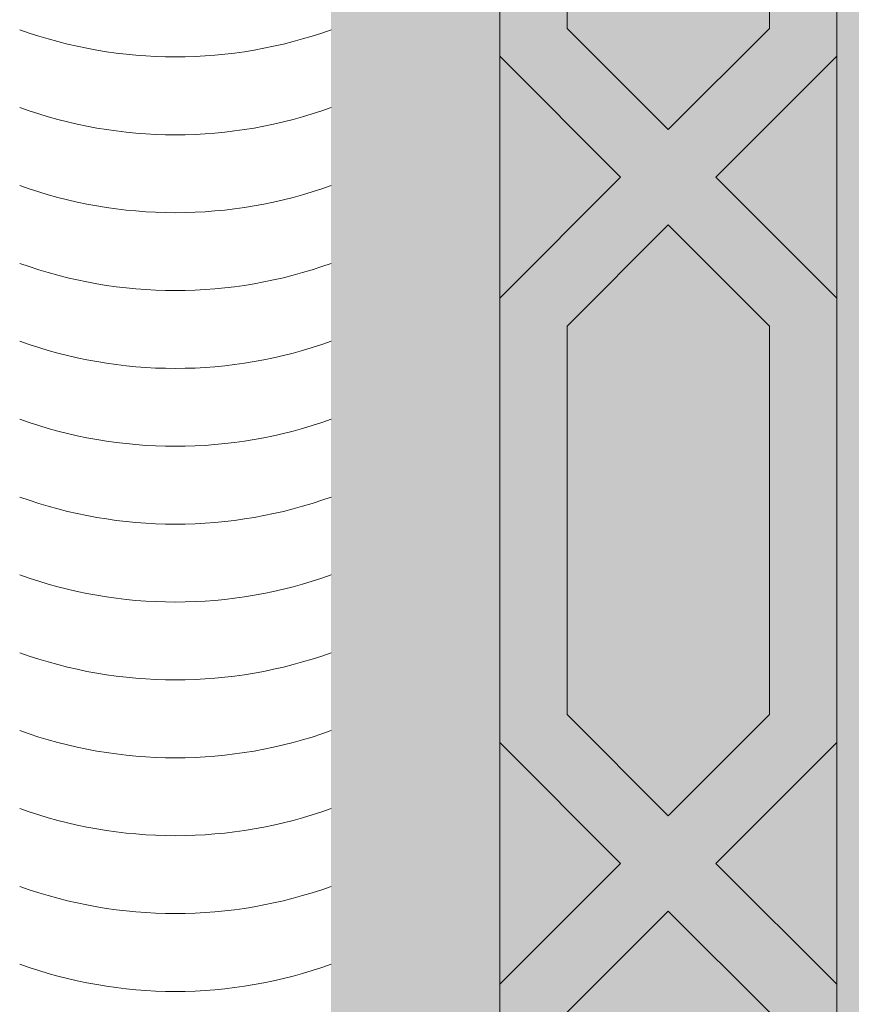
# Model space of a CAD drawing. Units: inches. Extents: x 844 to 2234, y 346 to 1084.
# Tile 58 of 93: x 1861.148 to 1864.294, y 706.48 to 710.205. Entities that reach past the tile are written whole.
import ezdxf

# ---------------------------------------------------------------- set-up
doc = ezdxf.new("R2010")
doc.units = ezdxf.units.IN
doc.header["$MEASUREMENT"] = 0
doc.layers.add('furniture', color=8, linetype='Continuous', lineweight=18)
doc.layers.add('RA-AP-01$0$INT', color=35, linetype='Continuous', lineweight=5)
doc.layers.add('RA-AP-01$0$FURN', color=3, linetype='Continuous')

# ---------------------------------------------------------------- blocks, each defined once
blk = doc.blocks.new('A$C18D01794')
at = {"layer": 'RA-AP-01$0$INT'}
h = blk.add_hatch(color=256, dxfattribs=at)
h.paths.add_polyline_path([(4.355206456958071, -6.156712009588037), (4.355206456958071, -8.056712009588038), (5.455206456958072, -8.056712009588038), (5.455206456958072, -6.156712009588037)])
h.paths.add_polyline_path([(4.405206456958072, -8.006712009588039), (4.405206456958072, -6.206712009588038), (5.405206456958072, -6.206712009588038), (5.405206456958072, -8.006712009588039)], flags=16)
h = blk.add_hatch(color=256, dxfattribs=at)
h.paths.add_polyline_path([(4.505206456958071, -7.585498806127123), (4.46934859260189, -7.549640941759413), (4.505206456958071, -7.513783077414768), (4.505206456958071, -7.381963272220687), (4.469348592616735, -7.346105407867824), (4.505206456958071, -7.310247543514964), (4.505206456958071, -7.178427738324996), (4.469348592586679, -7.142569873965138), (4.505206456952245, -7.106712009588038), (4.476922185709333, -7.106712009588038), (4.455206456960671, -7.128427738343681), (4.433490728198047, -7.106712009588038), (4.405206456946033, -7.106712009588036), (4.441064321339216, -7.142569873969684), (4.40520645695807, -7.178427738362358), (4.405206456958072, -7.310247543472698), (4.441064321364728, -7.346105407867826), (4.40520645695807, -7.381963272262947), (4.40520645695807, -7.513783077378263), (4.441064321354429, -7.549640941786153), (4.405206456958072, -7.585498806170974), (4.405206456958072, -7.717318611286652), (4.441064321333084, -7.753176475673194), (4.405206456958072, -7.789034340036673), (4.405206456958072, -8.006712009588039), (4.644348592588106, -8.006712009588039), (4.680206456964639, -7.970854145211967), (4.716064321341165, -8.006712009588039), (4.869348592586113, -8.006712009588039), (4.905206456964143, -7.970854145210465), (4.941064321342174, -8.006712009588039), (5.094348592587118, -8.006712009588037), (5.130206456963649, -7.970854145211967), (5.166064321340178, -8.006712009588039), (5.405206456958072, -8.006712009588039), (5.405206456958072, -7.789034340024526), (5.369348592595202, -7.753176475673196), (5.40520645695807, -7.717318611298797), (5.40520645695807, -7.585498806158829), (5.369348592573859, -7.549640941786151), (5.40520645695807, -7.51378307739041), (5.40520645695807, -7.381963272250803), (5.36934859256356, -7.346105407867824), (5.405206456958072, -7.310247543484846), (5.405206456958072, -7.178427738350217), (5.369348592589068, -7.142569873969682), (5.405206456982249, -7.106712009588038), (5.376922185730244, -7.106712009588038), (5.355206456967613, -7.128427738343679), (5.333490728218955, -7.10671200958804), (5.305206456976043, -7.106712009588042), (5.341064321341609, -7.142569873965136), (5.305206456958072, -7.178427738337141), (5.305206456958072, -7.310247543502816), (5.34106432131155, -7.346105407867824), (5.305206456958072, -7.381963272232832), (5.30520645695807, -7.513783077402624), (5.341064321326395, -7.549640941759413), (5.305206456958072, -7.585498806139263), (5.305206456958072, -7.717318611299605), (5.341064321347738, -7.753176475677737), (5.305206456958072, -7.78903434007894), (5.30520645695807, -7.906712009588039), (5.166064321336834, -7.906712009588039), (5.130206456963647, -7.942569873961684), (5.094348592590464, -7.906712009588039), (4.941064321338827, -7.906712009588041), (4.905206456964145, -7.942569873963183), (4.869348592589459, -7.906712009588039), (4.716064321337822, -7.906712009588041), (4.680206456964641, -7.942569873961684), (4.644348592591453, -7.906712009588039), (4.505206456958071, -7.906712009588039), (4.505206456958071, -7.789034340066795), (4.469348592580545, -7.753176475677738), (4.505206456958071, -7.717318611311748)])
h.paths.add_polyline_path([(4.485206456974132, -7.709034340046354), (4.45520645695909, -7.739034340051736), (4.425206456974128, -7.709034340057131), (4.425206456993394, -7.593783077384998), (4.45520645699153, -7.563783077396511), (4.485206456993396, -7.593783077408017)], flags=16)
h.paths.add_polyline_path([(4.455206456954537, -7.767318611299197), (4.485206456958242, -7.797318611312542), (4.48520645695951, -7.912569873958716), (4.45520645695415, -7.942569873954422), (4.425206456957888, -7.912569873967813), (4.425206456957888, -7.797318611286197)], flags=16)
h.paths.add_polyline_path([(4.455206456964794, -7.535498806149051), (4.42520645696469, -7.5054988061393), (4.425206456983954, -7.390247543486406), (4.455206456990734, -7.360247543489279), (4.485206456983953, -7.39024754349214), (4.485206456964687, -7.505498806158811)], flags=16)
h.paths.add_polyline_path([(4.499348592588947, -7.926712009585049), (4.636064321340932, -7.926712009585049), (4.666064321342317, -7.956712009586821), (4.636064321343707, -7.986712009585048), (4.499348592575121, -7.986712009585048), (4.469348592591685, -7.956712009591957)], flags=16)
h.paths.add_polyline_path([(4.425206456957888, -7.940854145195974), (4.471064321332215, -7.986712009585049), (4.425206456957888, -7.986712009585049)], flags=16)
h.paths.add_polyline_path([(4.455206456990734, -7.331963272246367), (4.425206456989053, -7.301963272254337), (4.425206456969784, -7.186712009596224), (4.455206456965226, -7.156712009591144), (4.485206456969787, -7.186712009586051), (4.485206456989053, -7.301963272238404)], flags=16)
h.paths.add_polyline_path([(4.72434859258714, -7.926712009586255), (4.861064321340141, -7.926712009586248), (4.891064321340324, -7.956712009586823), (4.861064321340513, -7.986712009586252), (4.724348592586768, -7.986712009586252), (4.694348592586956, -7.956712009586821)], flags=16)
h.paths.add_polyline_path([(4.919348592587961, -7.956712009586821), (4.949348592588145, -7.92671200958625), (5.08606432134115, -7.926712009586253), (5.116064321341327, -7.956712009586823), (5.086064321341519, -7.986712009586252), (4.949348592587774, -7.986712009586252)], flags=16)
h.paths.add_polyline_path([(5.144348592585967, -7.956712009586823), (5.174348592587358, -7.926712009585049), (5.311064321339338, -7.926712009585049), (5.3410643213366, -7.956712009591957), (5.311064321353163, -7.986712009585048), (5.174348592584576, -7.986712009585048)], flags=16)
h.paths.add_polyline_path([(5.32520645693489, -7.593783077408021), (5.355206456936755, -7.563783077396511), (5.385206456934894, -7.593783077384998), (5.38520645695416, -7.709034340057128), (5.355206456969194, -7.739034340051736), (5.325206456954153, -7.709034340046352)], flags=16)
h.paths.add_polyline_path([(5.325206456970042, -7.797318611312542), (5.355206456973747, -7.767318611299197), (5.385206456970398, -7.7973186112862), (5.385206456970398, -7.912569873967816), (5.355206456974136, -7.942569873954422), (5.325206456968778, -7.912569873958716)], flags=16)
h.paths.add_polyline_path([(5.325206456963599, -7.505498806158811), (5.325206456944333, -7.39024754349214), (5.355206456937552, -7.360247543489279), (5.385206456944332, -7.39024754348641), (5.385206456963596, -7.505498806139303), (5.355206456963492, -7.53549880614905)], flags=16)
h.paths.add_polyline_path([(5.32520645693923, -7.301963272238403), (5.3252064569585, -7.186712009586051), (5.355206456963062, -7.156712009591142), (5.3852064569585, -7.186712009596224), (5.385206456939234, -7.301963272254338), (5.355206456937552, -7.331963272246369)], flags=16)
h.paths.add_polyline_path([(5.339348592596071, -7.986712009585048), (5.385206456970398, -7.940854145195972), (5.385206456970396, -7.986712009585048)], flags=16)
h = blk.add_hatch(color=256, dxfattribs=at)
h.paths.add_polyline_path([(4.469348592586677, -7.142569873965136), (4.505206456958073, -7.178427738324996), (4.505206456958071, -7.106712009582215)])
h.paths.add_polyline_path([(4.455206456960671, -7.128427738343681), (4.476922185709333, -7.106712009588038), (4.433490728198045, -7.106712009588038)])
h.paths.add_polyline_path([(4.405206456958073, -7.178427738362358), (4.441064321339218, -7.142569873969684), (4.40520645695807, -7.106712009600073)])
h.paths.add_polyline_path([(4.425206456989053, -7.301963272254335), (4.455206456990736, -7.331963272246371), (4.485206456989055, -7.301963272238399), (4.48520645696979, -7.186712009586054), (4.455206456965227, -7.15671200959114), (4.425206456969784, -7.186712009596224)])
h.paths.add_polyline_path([(4.505206456958073, -7.381963272220689), (4.505206456958071, -7.310247543514961), (4.469348592616738, -7.346105407867826)])
h.paths.add_polyline_path([(4.425206456964688, -7.5054988061393), (4.455206456964794, -7.535498806149051), (4.485206456964689, -7.505498806158811), (4.485206456983951, -7.390247543492138), (4.455206456990736, -7.360247543489277), (4.425206456983956, -7.39024754348641)])
h.paths.add_polyline_path([(4.425206456974126, -7.709034340057128), (4.455206456959092, -7.739034340051736), (4.485206456974132, -7.709034340046356), (4.485206456993396, -7.593783077408017), (4.45520645699153, -7.563783077396511), (4.425206456993394, -7.593783077384999)])
h.paths.add_polyline_path([(4.46934859260189, -7.549640941759415), (4.505206456958071, -7.585498806127123), (4.505206456958073, -7.513783077414766)])
h.paths.add_polyline_path([(4.405206456958073, -7.585498806170972), (4.441064321354427, -7.549640941786151), (4.405206456958072, -7.513783077378263)])
h.paths.add_polyline_path([(4.405206456958072, -7.789034340036673), (4.441064321333084, -7.753176475673194), (4.405206456958072, -7.71731861128665)])
h.paths.add_polyline_path([(4.469348592580547, -7.75317647567774), (4.505206456958071, -7.789034340066795), (4.505206456958071, -7.717318611311744)])
h.paths.add_polyline_path([(4.425206456957888, -7.912569873967814), (4.45520645695415, -7.942569873954422), (4.485206456959507, -7.912569873958718), (4.48520645695824, -7.797318611312542), (4.455206456954537, -7.767318611299197), (4.425206456957888, -7.797318611286202)])
h.paths.add_polyline_path([(4.425206456957888, -7.986712009585049), (4.471064321332215, -7.986712009585049), (4.425206456957888, -7.940854145195972)])
h.paths.add_polyline_path([(4.499348592575121, -7.986712009585048), (4.636064321343707, -7.986712009585049), (4.666064321342317, -7.956712009586823), (4.636064321340932, -7.926712009585049), (4.499348592588945, -7.926712009585049), (4.469348592591685, -7.95671200959196)])
h.paths.add_polyline_path([(4.680206456964641, -7.942569873961684), (4.716064321337824, -7.906712009588039), (4.644348592591454, -7.906712009588039)])
h.paths.add_polyline_path([(4.644348592588108, -8.006712009588039), (4.716064321341167, -8.006712009588039), (4.680206456964637, -7.970854145211964)])
h.paths.add_polyline_path([(4.724348592586768, -7.98671200958625), (4.861064321340514, -7.986712009586252), (4.891064321340324, -7.956712009586819), (4.861064321340141, -7.92671200958625), (4.724348592587134, -7.926712009586255), (4.694348592586957, -7.956712009586821)])
h.paths.add_polyline_path([(4.905206456964143, -7.942569873963183), (4.941064321338827, -7.906712009588039), (4.869348592589457, -7.906712009588037)])
h.paths.add_polyline_path([(4.869348592586113, -8.006712009588039), (4.941064321342172, -8.006712009588037), (4.905206456964145, -7.970854145210463)])
h.paths.add_polyline_path([(4.949348592587774, -7.986712009586252), (5.086064321341521, -7.986712009586252), (5.116064321341329, -7.956712009586823), (5.08606432134115, -7.926712009586253), (4.949348592588145, -7.92671200958625), (4.919348592587961, -7.956712009586819)])
h.paths.add_polyline_path([(5.130206456963645, -7.942569873961684), (5.166064321336834, -7.906712009588039), (5.094348592590464, -7.906712009588039)])
h.paths.add_polyline_path([(5.094348592587119, -8.006712009588039), (5.166064321340178, -8.006712009588039), (5.130206456963651, -7.970854145211967)])
h.paths.add_polyline_path([(5.174348592584578, -7.986712009585048), (5.311064321353163, -7.986712009585048), (5.341064321336602, -7.956712009591958), (5.31106432133934, -7.926712009585049), (5.174348592587352, -7.926712009585049), (5.144348592585969, -7.956712009586823)])
h.paths.add_polyline_path([(5.325206456968778, -7.912569873958718), (5.355206456974136, -7.942569873954422), (5.385206456970396, -7.912569873967814), (5.385206456970396, -7.797318611286199), (5.355206456973747, -7.767318611299197), (5.325206456970044, -7.797318611312544)])
h.paths.add_polyline_path([(5.339348592596073, -7.986712009585048), (5.385206456970396, -7.986712009585049), (5.385206456970398, -7.94085414519597)])
h.paths.add_polyline_path([(5.325206456954155, -7.709034340046354), (5.355206456969194, -7.739034340051734), (5.38520645695416, -7.709034340057128), (5.385206456934896, -7.593783077384999), (5.355206456936758, -7.563783077396513), (5.325206456934888, -7.593783077408019)])
h.paths.add_polyline_path([(5.305206456958072, -7.789034340078938), (5.341064321347739, -7.753176475677738), (5.305206456958072, -7.717318611299605)])
h.paths.add_polyline_path([(5.369348592595204, -7.753176475673194), (5.40520645695807, -7.789034340024526), (5.405206456958072, -7.717318611298798)])
h.paths.add_polyline_path([(5.405206456958072, -7.585498806158831), (5.405206456958072, -7.513783077390407), (5.369348592573857, -7.549640941786151)])
h.paths.add_polyline_path([(5.305206456958072, -7.585498806139266), (5.341064321326393, -7.549640941759413), (5.305206456958072, -7.513783077402626)])
h.paths.add_polyline_path([(5.325206456963599, -7.50549880615881), (5.355206456963494, -7.535498806149055), (5.385206456963598, -7.505498806139302), (5.385206456944334, -7.390247543486411), (5.355206456937552, -7.360247543489279), (5.325206456944333, -7.39024754349214)])
h.paths.add_polyline_path([(5.305206456958072, -7.38196327223283), (5.341064321311551, -7.346105407867824), (5.305206456958072, -7.31024754350282)])
h.paths.add_polyline_path([(5.325206456939231, -7.301963272238404), (5.355206456937552, -7.331963272246369), (5.385206456939235, -7.301963272254335), (5.385206456958502, -7.186712009596224), (5.355206456963061, -7.156712009591142), (5.3252064569585, -7.186712009586051)])
h.paths.add_polyline_path([(5.404581768715993, -7.381338584008926, -0.001217816984214), (5.405206456958072, -7.381112009582329), (5.405206456958072, -7.310247543484846), (5.369348592563558, -7.346105407867826)])
h.paths.add_polyline_path([(5.36934859258907, -7.142569873969684), (5.40520645695807, -7.178427738350215), (5.405206456958072, -7.106712009612218)])
h.paths.add_polyline_path([(5.355206456967613, -7.128427738343683), (5.376922185730239, -7.106712009588038), (5.333490728218953, -7.10671200958804)])
h.paths.add_polyline_path([(5.30520645695807, -7.178427738337139), (5.341064321341609, -7.142569873965134), (5.305206456958074, -7.10671200957007)])
blk.add_hatch(color=256, dxfattribs=at).paths.add_polyline_path([(4.505206456958071, -7.906712009588039), (5.305206456958072, -7.906712009588039), (5.305206456958072, -7.106712009588038), (5.255206456951893, -7.106712009588036), (5.25520645694868, -7.856712009570104), (4.555206456959269, -7.856712009588616), (4.555206456956052, -7.106712009588038), (4.505206456958073, -7.106712009588038)])
for p, q in [((4.425206456964688, -7.5054988061393), (4.455206456964796, -7.535498806149051)), ((4.485206456964687, -7.505498806158811), (4.455206456964796, -7.535498806149051)), ((4.405206456968717, -7.513783077388909), (4.441064321338788, -7.54964094177051)), ((4.505206456968717, -7.513783077404122), (4.469348592586251, -7.549640941775054)), ((4.405206456988469, -7.585498806140577), (4.441064321370071, -7.549640941770508)), ((4.505206456988468, -7.58549880615752), (4.469348592617532, -7.549640941775056)), ((4.425206456993394, -7.593783077384996), (4.45520645699153, -7.563783077396511)), ((4.485206456993396, -7.593783077408017), (4.45520645699153, -7.563783077396511)), ((4.425206456993394, -7.593783077384996), (4.425206456974128, -7.709034340057129)), ((4.485206456993396, -7.593783077408017), (4.485206456974132, -7.709034340046354)), ((4.425206456974128, -7.709034340057129), (4.455206456959092, -7.739034340051736)), ((4.485206456974132, -7.709034340046354), (4.455206456959092, -7.739034340051736)), ((4.405206456963013, -7.717318611291593), (4.441064321333084, -7.753176475673194)), ((4.505206456963013, -7.717318611306806), (4.469348592580547, -7.753176475677738)), ((4.441064321333084, -7.753176475673194), (4.405206456950156, -7.789034340044587)), ((4.469348592580547, -7.753176475677738), (4.505206456951941, -7.789034340060664)), ((4.455206456954537, -7.767318611299197), (4.425206456957888, -7.797318611286199)), ((4.455206456954537, -7.767318611299197), (4.485206456958242, -7.797318611312544)), ((4.425206456957888, -7.797318611286199), (4.425206456957888, -7.912569873967814)), ((4.485206456959509, -7.912569873958718), (4.485206456958242, -7.797318611312544))]:
    blk.add_line(p, q, dxfattribs=at)
for points in [[(5.405206456958072, -8.006712009588039), (4.405206456958072, -8.006712009588039), (4.405206456958072, -7.106712009588038)], [(5.305206456958072, -7.106712009588038), (5.305206456958072, -7.906712009588039), (4.505206456958071, -7.906712009588039), (4.505206456958071, -7.106712009588038)]]:
    blk.add_lwpolyline(points, dxfattribs=at)
for centre in [(4.309006456954359, -7.648064458284158), (4.309006456951176, -7.671164458284799), (4.309006456954132, -7.671164458285863), (4.309006456953905, -7.694264458283548), (4.309006456953905, -7.717364458282297), (4.309006456952313, -7.740464458286957), (4.30900645695345, -7.763564458285706), (4.30900645695345, -7.786664458281272), (4.309006456951858, -7.80976445828616), (4.309006456950039, -7.832864458284682), (4.309006456952995, -7.855964458280475), (4.309006456952768, -7.879064458285135), (4.309006456951176, -7.902164458283884), (4.309006456949584, -7.925264458285589)]:
    blk.add_arc(centre, 0.136414042854523, 70.20384312815696, 109.7961568705686, dxfattribs=at)
blk = doc.blocks.new('A$C5D2F253E')
at = {"layer": 'RA-AP-01$0$FURN', "xscale": -0.7999999999883585, "yscale": 0.7999999999883585, "zscale": 0.8, "rotation": 90}
blk.add_blockref('A$C18D01794', (-5.687757199772477, 4.75791982714071), dxfattribs=at)

msp = doc.modelspace()

# ---------------------------------------------------------------- block references
at = {"layer": 'furniture', "xscale": 15.94108302203742, "yscale": 15.94108302203742, "zscale": 15.94108302203742, "rotation": 90}
msp.add_blockref('A$C5D2F253E', (1882.631064852549, 701.4028671565849), dxfattribs=at)

doc.saveas('drawing.dxf')
